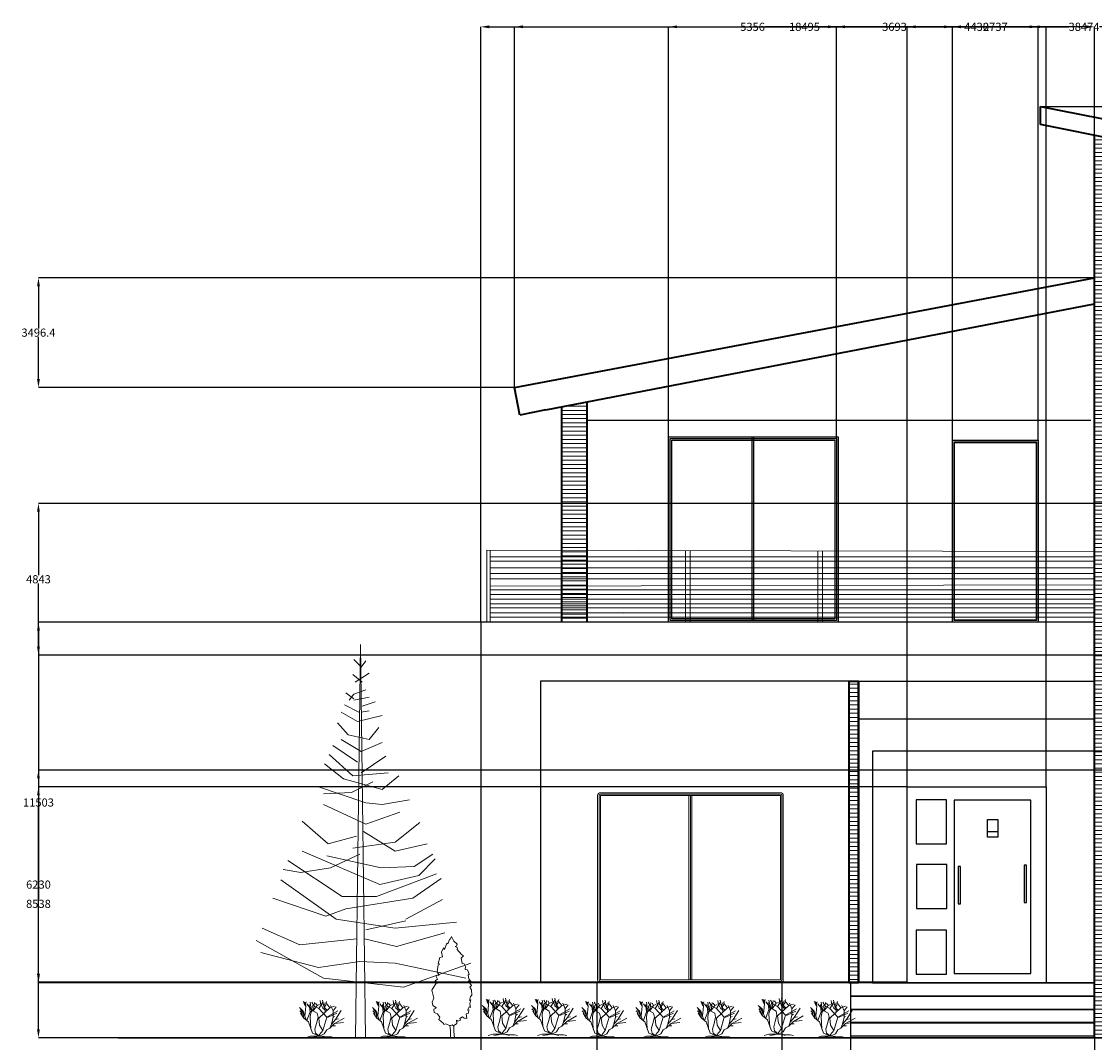
# Model space of a CAD drawing. Units: millimetres. Extents: x 23 to 3809233, y 4 to 290343.
# Tile 7 of 8: x 1887648 to 1921861, y 173128 to 205695. Entities that reach past the tile are written whole.
import ezdxf

# ---------------------------------------------------------------- set-up
doc = ezdxf.new("R2010")
doc.units = ezdxf.units.MM
doc.header["$MEASUREMENT"] = 0
for name, color, linetype, lineweight in [('A-ANNO-DIMS', 2, 'Continuous', 18), ('A-COLS', 7, 'Continuous', 35), ('A-DOOR', 3, 'Continuous', 25), ('A-ELEV', 7, 'Continuous', 25), ('A-ELEV-GRND', 7, 'Continuous', 30), ('A-FLOR-RAIL', 8, 'Continuous', 18), ('A-FLOR-STRS', 7, 'Continuous', 25), ('A-GLAZ', 4, 'Continuous', 18), ('A-ROOF', 7, 'Continuous', 35), ('A-WALL-PATT', 252, 'Continuous', 13), ('L-PLNT', 94, 'Continuous', 13)]:
    doc.layers.add(name, color=color, linetype=linetype, lineweight=lineweight)
doc.styles.get("Standard").update_dxf_attribs({"font": 'arial.ttf'})
doc.dimstyles.get("Standard").update_dxf_attribs({"dimtxt": 260.18, "dimasz": 270.18, "dimexe": 0.18, "dimexo": 0.0625, "dimgap": 0.09, "dimtad": 0, "dimtih": 1, "dimtoh": 1, "dimdec": 0, "dimzin": 0, "dimdsep": 46, "dimtxsty": 'Standard', "dimcen": 0.09, "dimadec": 0, "dimazin": 0, "dimtfac": 1, "dimtdec": 0, "dimtofl": 0, "dimtmove": 0, "dimatfit": 3, "dimfxl": 1, "dimtolj": 1, "dimtzin": 0, "dimarcsym": 0})

# ---------------------------------------------------------------- blocks, each defined once
blk = doc.blocks.new('*U6')
blk.add_lwpolyline([(-2.754, 191.699), (-6.78, 182.851), (-13.682, 176.953), (-11.956, 173.266), (-9.656, 172.529), (-14.257, 170.317), (-13.682, 167.368), (-21.733, 157.783), (-25.184, 154.834), (-21.158, 150.41), (-21.733, 147.461), (-22.884, 140.825), (-26.334, 140.087), (-29.21, 134.926), (-28.635, 129.028), (-32.661, 128.291), (-36.111, 120.18), (-34.386, 118.706), (-35.536, 111.333), (-38.987, 106.171), (-34.386, 107.646), (-40.712, 98.798), (-37.261, 95.849), (-40.712, 90.688), (-41.287, 80.366), (-38.412, 78.154), (-36.686, 70.781), (-39.562, 71.518), (-37.261, 64.145), (-38.412, 57.509), (-36.111, 58.247), (-33.236, 52.348), (-35.536, 53.086), (-34.961, 46.45), (-30.36, 44.975), (-31.51, 36.128), (-26.334, 36.865), (-23.459, 39.814), (-18.283, 36.128), (-20.008, 33.178), (-14.832, 31.704), (-11.956, 33.178), (-12.531, 27.28), (-6.205, 22.856), (-3.905, 24.331), (0.121, 22.856), (8.173, 26.543), (11.624, 25.068), (12.199, 27.28), (21.4, 34.653), (19.675, 39.077), (23.701, 44.975), (30.027, 47.924), (30.602, 53.823), (25.426, 56.772), (32.903, 61.196), (34.053, 67.094), (30.602, 75.205), (34.628, 89.951), (26.576, 103.222), (23.701, 103.222), (28.302, 107.646), (23.701, 110.595), (26.576, 115.756), (25.426, 117.968), (20.825, 118.706), (24.276, 124.604), (22.551, 137.876), (19.1, 139.35), (22.551, 140.825), (19.675, 151.884), (14.499, 153.359), (16.224, 162.207), (12.199, 170.317), (10.473, 167.368), (5.872, 179.165), (4.147, 177.69), (0.696, 187.275), (-0.454, 185.8)], close=True)
for points in [[(-6.813, 23.669), (-6.813, 11.669), (-8.627, 0)], [(0.387, 23.669), (-0.576, 13.271), (-0.576, 3.686), (0, 0)]]:
    blk.add_lwpolyline(points)
blk = doc.blocks.new('*U8')
for p, q in [((-2.401, 192), (-4.8, 0)), ((-2.401, 192), (0, 0)), ((-4.988, 183.92), (-2.688, 180.971)), ((-3.263, 186.869), (0.188, 186.869)), ((-2.113, 181.708), (0.763, 184.657)), ((-6.714, 178.022), (0.188, 173.598)), ((-3.263, 173.598), (1.338, 177.284)), ((-4.988, 169.911), (0.763, 167.699)), ((0.763, 165.487), (4.788, 168.437)), ((0.763, 167.699), (3.063, 164.75)), ((-3.263, 161.801), (-9.59, 164.013)), ((-6.714, 166.225), (0.763, 164.75)), ((-1.538, 158.852), (5.364, 162.538)), ((-0.963, 154.428), (-13.04, 157.377)), ((-6.714, 159.589), (-2.688, 158.852)), ((7.089, 158.852), (-0.963, 154.428)), ((-42.371, 67.426), (-24.542, 57.841)), ((-24.542, 57.104), (-4.988, 52.68)), ((27.218, 45.307), (45.622, 53.417)), ((-43.521, 51.205), (-19.942, 44.569)), ((-19.942, 44.569), (-4.413, 48.256)), ((-0.388, 48.256), (27.218, 45.307))]:
    blk.add_line(p, q)
for points in [[(8.814, 153.691), (3.638, 147.792), (-6.714, 145.58), (-11.315, 151.479)], [(-13.04, 144.106), (-2.688, 139.682), (7.089, 145.58)], [(-0.963, 134.521), (11.115, 142.631)], [(-15.916, 129.36), (1.338, 127.885), (12.84, 138.207)], [(-14.766, 137.47), (-2.688, 129.36)], [(-21.092, 127.885), (-13.04, 121.249), (5.939, 126.41), (15.141, 133.783)], [(-26.268, 116.088), (-13.04, 113.876), (-4.988, 114.613), (18.591, 122.724)], [(-8.439, 124.936), (1.913, 119.775), (15.716, 119.037)], [(-21.667, 110.19), (-4.988, 104.291), (15.716, 113.876)], [(-31.444, 105.028), (-19.366, 95.443), (1.338, 92.494)], [(-0.388, 98.393), (13.415, 94.706), (26.068, 105.766)], [(-34.895, 94.706), (-19.366, 91.02), (-3.838, 100.605)], [(-38.92, 87.333), (-30.869, 79.223), (-11.89, 74.799), (26.068, 91.02)], [(-37.77, 89.545), (-28.568, 83.647), (-12.465, 82.909), (13.99, 88.808)], [(-2.113, 89.545), (12.265, 82.909), (26.643, 80.697), (35.27, 82.172)], [(-39.496, 79.96), (-10.165, 68.901), (6.514, 68.901), (32.969, 86.596)], [(-49.272, 56.366), (-19.366, 53.417), (9.389, 57.841), (36.42, 77.011)], [(-41.796, 77.748), (-27.993, 68.163), (4.788, 63.002), (14.565, 59.316), (40.446, 68.163)], [(-56.174, 36.459), (-23.392, 24.662), (15.716, 29.086), (48.497, 47.519)], [(-53.873, 29.086), (-19.366, 36.459), (-2.113, 37.196), (18.016, 34.247), (46.197, 41.62)]]:
    blk.add_lwpolyline(points)
blk = doc.blocks.new('*U7')
for p, q in [((-16.8, 16.32), (-15.36, 19.68)), ((-14.88, 18.24), (-12.96, 20.64)), ((-12.471, 19.775), (-12.898, 22.044)), ((-11.677, 19.071), (-12.471, 19.775)), ((-11.28, 19.619), (-12.104, 21.184)), ((-11.921, 18.836), (-10.64, 20.401)), ((-11.433, 18.289), (-10.457, 22.749)), ((-10.579, 18.054), (-9.846, 19.697)), ((-8.16, 17.76), (-10.56, 21.6)), ((-9.48, 19.775), (-8.992, 22.592)), ((-7.2, 19.68), (-8.64, 20.16)), ((-7.2, 19.68), (-6.24, 21.12)), ((-4.8, 16.32), (-7.2, 19.68)), ((-5.086, 17.741), (-5.513, 21.34)), ((-5.28, 19.2), (-3.84, 21.6)), ((-2.88, 12.96), (-4.32, 19.68)), ((-3.84, 16.8), (-0.96, 20.64)), ((-3.377, 18.602), (-2.888, 21.575)), ((-2.88, 15.84), (-2.4, 20.16)), ((-0.508, 21.888), (-0.081, 20.558)), ((-0.203, 19.149), (0.102, 21.34)), ((-0.142, 19.384), (0.59, 20.401)), ((-0.02, 20.01), (0.896, 21.105)), ((0.041, 20.714), (1.384, 22.044)), ((0.102, 21.34), (0.835, 21.888)), ((-18.24, 11.04), (-21.755, 16.655)), ((-12.96, 12.48), (-19.68, 16.32)), ((-13.92, 12.48), (-19.2, 14.88)), ((-16.8, 16.32), (-18.72, 18.72)), ((-14.88, 18.24), (-17.76, 19.2)), ((-16.8, 12.48), (-16.8, 16.32)), ((-8.16, 12), (-14.88, 18.24)), ((-13.325, 16.724), (-11.433, 18.289)), ((-12.96, 12.48), (-8.16, 17.76)), ((-12.043, 15.628), (-11.921, 18.836)), ((-11.982, 16.802), (-10.579, 18.054)), ((-8.16, 17.76), (-5.28, 19.2)), ((-7.68, 12.48), (-7.2, 14.88)), ((-7.2, 14.88), (-3.84, 16.8)), ((-3.377, 15.315), (-5.086, 17.819)), ((-2.766, 16.802), (-3.377, 18.602)), ((-0.96, 10.56), (-2.88, 15.84)), ((-0.48, 10.8), (0.346, 13.203)), ((0.346, 13.203), (-0.203, 19.149)), ((0.346, 13.203), (1.323, 16.254)), ((0.96, 12), (1.44, 15.36)), ((0.96, 12), (2.88, 14.88)), ((1.323, 16.254), (3.642, 18.289)), ((1.44, 15.36), (2.88, 17.28)), ((1.92, 13.44), (2.4, 15.36)), ((2.4, 15.36), (3.36, 16.32)), ((-17.76, 8.64), (-23.663, 11.961)), ((-17.76, 8.64), (-23.128, 9.222)), ((-18.24, 11.04), (-20.16, 11.52)), ((-15.84, 8.16), (-18.24, 11.04)), ((-16.32, 7.2), (-18.24, 7.2)), ((-16.8, 12.48), (-17.76, 12.96)), ((-14.88, 5.76), (-17.76, 8.64)), ((-15.84, 8.16), (-16.8, 12.48)), ((-14.88, 5.76), (-15.84, 8.16)), ((-12.96, 12.48), (-13.92, 12.48)), ((-10.56, 4.32), (-12.96, 12.48)), ((-10.56, 4.32), (-8.64, 7.68)), ((-8.64, 7.68), (-8.16, 12)), ((-6.72, 8.64), (-7.68, 12.48)), ((-5.76, 5.28), (-6.72, 8.64)), ((-4.32, 2.88), (-1.92, 9.6)), ((-3.36, 5.28), (-2.88, 12.96)), ((-1.92, 9.6), (0.96, 12)), ((-15.84, 0.48), (-17.76, 0)), ((-13.44, 0.48), (-15.84, 0.48)), ((-12.96, 4.8), (-14.88, 5.76)), ((-9.6, 0.96), (-13.44, 0.48)), ((-11.52, 2.4), (-12.96, 4.8)), ((-9.6, 0.96), (-12.96, 0)), ((-8.64, 0.96), (-11.52, 2.4)), ((-8.64, 1.92), (-10.56, 4.32)), ((-9.6, 0.96), (-7.68, 0.96)), ((-8.64, 0.96), (-4.32, 2.88)), ((-8.64, 0.96), (-6.24, 2.88)), ((-8.64, 0.96), (-8.64, 1.92)), ((-8.64, 0.96), (-2.88, 0.96)), ((-7.68, 0.96), (-6.24, 0.48)), ((-6.24, 2.88), (-5.76, 5.28)), ((-6.24, 0.48), (-3.36, 0)), ((-2.88, 0.96), (0, 0))]:
    blk.add_line(p, q)
blk = doc.blocks.new('*D94')
at = {"layer": 'A-ANNO-DIMS', "color": 0, "lineweight": -2, "transparency": 16777216}
for p, q in [((1902289, 186535), (1902289, 205525)), ((1902560, 205524), (1921037, 205524)), ((1940493, 205524), (1922015, 205524)), ((1940763, 198959), (1940763, 205525))]:
    blk.add_line(p, q, dxfattribs=at)
at = {"layer": 'A-ANNO-DIMS', "color": 0, "transparency": 16777216}
for points in [[(1902560, 205569), (1902560, 205479), (1902289, 205524)], [(1940493, 205569), (1940493, 205479), (1940763, 205524)]]:
    blk.add_solid(points, dxfattribs=at)
at = {"layer": 'Defpoints', "color": 0, "transparency": 16777216}
for p in [(1940763, 205524), (1940763, 198959), (1902289, 186535)]:
    blk.add_point(p, dxfattribs=at)
at = {"layer": 'A-ANNO-DIMS', "color": 0, "transparency": 16777216, "insert": (1921526, 205524), "char_height": 260.2, "attachment_point": 5}
blk.add_mtext('\\A1;38474', dxfattribs=at)
blk = doc.blocks.new('*D95')
at = {"layer": 'A-ANNO-DIMS', "color": 0, "lineweight": -2, "transparency": 16777216}
for p, q in [((1920137, 202978), (1944019, 202978)), ((1944019, 202708), (1944019, 188263)), ((1944019, 173551), (1944019, 187997)), ((1939891, 173281), (1944019, 173281))]:
    blk.add_line(p, q, dxfattribs=at)
at = {"layer": 'A-ANNO-DIMS', "color": 0, "transparency": 16777216}
for points in [[(1943974, 202708), (1944064, 202708), (1944019, 202978)], [(1943974, 173551), (1944064, 173551), (1944019, 173281)]]:
    blk.add_solid(points, dxfattribs=at)
at = {"layer": 'Defpoints', "color": 0, "transparency": 16777216}
for p in [(1920137, 202978), (1944019, 202978), (1939891, 173281)]:
    blk.add_point(p, dxfattribs=at)
at = {"layer": 'A-ANNO-DIMS', "color": 0, "transparency": 16777216, "insert": (1944019, 188130), "char_height": 260.2, "attachment_point": 5}
blk.add_mtext('\\A1;29698', dxfattribs=at)
blk = doc.blocks.new('*D96')
at = {"layer": 'A-ANNO-DIMS', "color": 0, "lineweight": -2, "transparency": 16777216}
for p, q in [((1902289, 175032), (1902289, 166038)), ((1905995, 175031), (1905995, 166038)), ((1902560, 166038), (1903754, 166038)), ((1905725, 166038), (1904531, 166038))]:
    blk.add_line(p, q, dxfattribs=at)
at = {"layer": 'A-ANNO-DIMS', "color": 0, "transparency": 16777216}
for points in [[(1902560, 166083), (1902560, 165993), (1902289, 166038)], [(1905725, 166083), (1905725, 165993), (1905995, 166038)]]:
    blk.add_solid(points, dxfattribs=at)
at = {"layer": 'Defpoints', "color": 0, "transparency": 16777216}
for p in [(1902289, 175032), (1905995, 175031), (1905995, 166038)]:
    blk.add_point(p, dxfattribs=at)
at = {"layer": 'A-ANNO-DIMS', "color": 0, "transparency": 16777216, "insert": (1904142, 166038), "char_height": 260.2, "attachment_point": 5}
blk.add_mtext('\\A1;3706', dxfattribs=at)
blk = doc.blocks.new('*D97')
at = {"layer": 'A-ANNO-DIMS', "color": 0, "lineweight": -2, "transparency": 16777216}
for p, q in [((1905995, 175031), (1905995, 166038)), ((1911896, 175048), (1911896, 166038)), ((1906265, 166038), (1908582, 166038)), ((1911626, 166038), (1909309, 166038))]:
    blk.add_line(p, q, dxfattribs=at)
at = {"layer": 'A-ANNO-DIMS', "color": 0, "transparency": 16777216}
for points in [[(1906265, 166083), (1906265, 165993), (1905995, 166038)], [(1911626, 166083), (1911626, 165993), (1911896, 166038)]]:
    blk.add_solid(points, dxfattribs=at)
at = {"layer": 'Defpoints', "color": 0, "transparency": 16777216}
for p in [(1905995, 175031), (1911896, 175048), (1911896, 166038)]:
    blk.add_point(p, dxfattribs=at)
at = {"layer": 'A-ANNO-DIMS', "color": 0, "transparency": 16777216, "insert": (1908945, 166038), "char_height": 260.2, "attachment_point": 5}
blk.add_mtext('\\A1;5901', dxfattribs=at)
blk = doc.blocks.new('*D98')
at = {"layer": 'A-ANNO-DIMS', "color": 0, "lineweight": -2, "transparency": 16777216}
for p, q in [((1911896, 175048), (1911896, 166038)), ((1914080, 175026), (1914080, 166038)), ((1912166, 166038), (1912598, 166038)), ((1913810, 166038), (1913378, 166038))]:
    blk.add_line(p, q, dxfattribs=at)
at = {"layer": 'A-ANNO-DIMS', "color": 0, "transparency": 16777216}
for points in [[(1912166, 166083), (1912166, 165993), (1911896, 166038)], [(1913810, 166083), (1913810, 165993), (1914080, 166038)]]:
    blk.add_solid(points, dxfattribs=at)
at = {"layer": 'Defpoints', "color": 0, "transparency": 16777216}
for p in [(1911896, 175048), (1914080, 175026), (1914080, 166038)]:
    blk.add_point(p, dxfattribs=at)
at = {"layer": 'A-ANNO-DIMS', "color": 0, "transparency": 16777216, "insert": (1912988, 166038), "char_height": 260.2, "attachment_point": 5}
blk.add_mtext('\\A1;2184', dxfattribs=at)
blk = doc.blocks.new('*D102')
at = {"layer": 'A-ANNO-DIMS', "color": 0, "lineweight": -2, "transparency": 16777216}
for p, q in [((1914079.851314, 175025.824019), (1914079.851314, 166037.51032)), ((1921856.95103, 175025.824019), (1921856.95103, 166037.51032)), ((1914350.031314, 166037.69032), (1917580.88079, 166037.69032)), ((1921586.77103, 166037.69032), (1918355.921554, 166037.69032))]:
    blk.add_line(p, q, dxfattribs=at)
at = {"layer": 'A-ANNO-DIMS', "color": 0, "transparency": 16777216}
for points in [[(1914350.031314, 166082.72032), (1914350.031314, 165992.66032), (1914079.851314, 166037.69032)], [(1921586.77103, 166082.72032), (1921586.77103, 165992.66032), (1921856.95103, 166037.69032)]]:
    blk.add_solid(points, dxfattribs=at)
at = {"layer": 'Defpoints', "color": 0, "transparency": 16777216}
for p in [(1914079.851314, 175025.886519), (1921856.95103, 175025.886519), (1921856.95103, 166037.69032)]:
    blk.add_point(p, dxfattribs=at)
at = {"layer": 'A-ANNO-DIMS', "color": 0, "transparency": 16777216, "insert": (1917968.401172, 166037.69032), "char_height": 260.18, "attachment_point": 5}
blk.add_mtext('\\A1;7777', dxfattribs=at)
blk = doc.blocks.new('*D103')
at = {"layer": 'A-ANNO-DIMS', "color": 0, "lineweight": -2, "transparency": 16777216}
for p, q in [((1902289.331647, 186534.824099), (1888189.886131, 186534.824099)), ((1888190.066131, 186264.644099), (1888190.066131, 180916.359871)), ((1888190.066131, 175302.036407), (1888190.066131, 180650.320635)), ((1902289.331647, 175031.856407), (1888189.886131, 175031.856407))]:
    blk.add_line(p, q, dxfattribs=at)
at = {"layer": 'A-ANNO-DIMS', "color": 0, "transparency": 16777216}
for points in [[(1888145.036131, 186264.644099), (1888235.096131, 186264.644099), (1888190.066131, 186534.824099)], [(1888145.036131, 175302.036407), (1888235.096131, 175302.036407), (1888190.066131, 175031.856407)]]:
    blk.add_solid(points, dxfattribs=at)
at = {"layer": 'Defpoints', "color": 0, "transparency": 16777216}
for p in [(1888190.066131, 186534.824099), (1902289.394147, 186534.824099), (1902289.394147, 175031.856407)]:
    blk.add_point(p, dxfattribs=at)
at = {"layer": 'A-ANNO-DIMS', "color": 0, "transparency": 16777216, "insert": (1888190.066131, 180783.340253), "char_height": 260.18, "attachment_point": 5}
blk.add_mtext('\\A1;11503', dxfattribs=at)
blk = doc.blocks.new('*D104')
at = {"layer": 'A-ANNO-DIMS', "color": 0, "lineweight": -2, "transparency": 16777216}
for p, q in [((1924370.307623, 181820.425276), (1888189.886131, 181820.425276)), ((1888190.066131, 181550.245276), (1888190.066131, 177684.406757)), ((1888190.066131, 173552.529002), (1888190.066131, 177418.367521)), ((1924370.346212, 173282.349002), (1888189.886131, 173282.349002))]:
    blk.add_line(p, q, dxfattribs=at)
at = {"layer": 'A-ANNO-DIMS', "color": 0, "transparency": 16777216}
for points in [[(1888145.036131, 181550.245276), (1888235.096131, 181550.245276), (1888190.066131, 181820.425276)], [(1888145.036131, 173552.529002), (1888235.096131, 173552.529002), (1888190.066131, 173282.349002)]]:
    blk.add_solid(points, dxfattribs=at)
at = {"layer": 'Defpoints', "color": 0, "transparency": 16777216}
for p in [(1888190.066131, 181820.425276), (1924370.370123, 181820.425276), (1924370.408712, 173282.349002)]:
    blk.add_point(p, dxfattribs=at)
at = {"layer": 'A-ANNO-DIMS', "color": 0, "transparency": 16777216, "insert": (1888190.066131, 177551.387139), "char_height": 260.18, "attachment_point": 5}
blk.add_mtext('\\A1;8538', dxfattribs=at)
blk = doc.blocks.new('*D105')
at = {"layer": 'A-ANNO-DIMS', "color": 0, "lineweight": -2, "transparency": 16777216}
for p, q in [((1903366, 194022), (1903366, 205525)), ((1903636, 205524), (1912135, 205524)), ((1921591, 205524), (1913092, 205524)), ((1921861, 197518), (1921861, 205525))]:
    blk.add_line(p, q, dxfattribs=at)
at = {"layer": 'A-ANNO-DIMS', "color": 0, "transparency": 16777216}
for points in [[(1903636, 205569), (1903636, 205479), (1903366, 205524)], [(1921591, 205569), (1921591, 205479), (1921861, 205524)]]:
    blk.add_solid(points, dxfattribs=at)
at = {"layer": 'Defpoints', "color": 0, "transparency": 16777216}
for p in [(1921861, 205524), (1921861, 197518), (1903366, 194022)]:
    blk.add_point(p, dxfattribs=at)
at = {"layer": 'A-ANNO-DIMS', "color": 0, "transparency": 16777216, "insert": (1912613, 205524), "char_height": 260.2, "attachment_point": 5}
blk.add_mtext('\\A1;18495', dxfattribs=at)
blk = doc.blocks.new('*D107')
at = {"layer": 'A-ANNO-DIMS', "color": 0, "lineweight": -2, "transparency": 16777216}
for p, q in [((1921861, 197518), (1888190, 197518)), ((1888190, 197248), (1888190, 195903)), ((1888190, 194292), (1888190, 195637)), ((1903366, 194022), (1888190, 194022))]:
    blk.add_line(p, q, dxfattribs=at)
at = {"layer": 'A-ANNO-DIMS', "color": 0, "transparency": 16777216}
for points in [[(1888145, 197248), (1888235, 197248), (1888190, 197518)], [(1888145, 194292), (1888235, 194292), (1888190, 194022)]]:
    blk.add_solid(points, dxfattribs=at)
at = {"layer": 'Defpoints', "color": 0, "transparency": 16777216}
for p in [(1888190, 197518), (1921861, 197518), (1903366, 194022)]:
    blk.add_point(p, dxfattribs=at)
at = {"layer": 'A-ANNO-DIMS', "color": 0, "transparency": 16777216, "insert": (1888190, 195770), "char_height": 260.2, "attachment_point": 5}
blk.add_mtext('\\A1;3496.4', dxfattribs=at)
blk = doc.blocks.new('*D108')
at = {"layer": 'A-ANNO-DIMS', "color": 0, "lineweight": -2, "transparency": 16777216}
for p, q in [((1915886, 181281), (1915886, 205525)), ((1916157, 205524), (1917708, 205524)), ((1920046, 205524), (1918495, 205524)), ((1920317, 181281), (1920317, 205525))]:
    blk.add_line(p, q, dxfattribs=at)
at = {"layer": 'A-ANNO-DIMS', "color": 0, "transparency": 16777216}
for points in [[(1916157, 205569), (1916157, 205479), (1915886, 205524)], [(1920046, 205569), (1920046, 205479), (1920317, 205524)]]:
    blk.add_solid(points, dxfattribs=at)
at = {"layer": 'Defpoints', "color": 0, "transparency": 16777216}
for p in [(1920317, 205524), (1915886, 181281), (1920317, 181281)]:
    blk.add_point(p, dxfattribs=at)
at = {"layer": 'A-ANNO-DIMS', "color": 0, "transparency": 16777216, "insert": (1918101, 205524), "char_height": 260.2, "attachment_point": 5}
blk.add_mtext('\\A1;4430', dxfattribs=at)
blk = doc.blocks.new('*D109')
at = {"layer": 'A-ANNO-DIMS', "color": 0, "lineweight": -2, "transparency": 16777216}
for p, q in [((1915886, 181281), (1888190, 181281)), ((1888190, 181011), (1888190, 178299)), ((1888190, 175321), (1888190, 178033)), ((1915875, 175051), (1888190, 175051))]:
    blk.add_line(p, q, dxfattribs=at)
at = {"layer": 'A-ANNO-DIMS', "color": 0, "transparency": 16777216}
for points in [[(1888145, 181011), (1888235, 181011), (1888190, 181281)], [(1888145, 175321), (1888235, 175321), (1888190, 175051)]]:
    blk.add_solid(points, dxfattribs=at)
at = {"layer": 'Defpoints', "color": 0, "transparency": 16777216}
for p in [(1888190, 181281), (1915886, 181281), (1915875, 175051)]:
    blk.add_point(p, dxfattribs=at)
at = {"layer": 'A-ANNO-DIMS', "color": 0, "transparency": 16777216, "insert": (1888190, 178166), "char_height": 260.2, "attachment_point": 5}
blk.add_mtext('\\A1;6230', dxfattribs=at)
blk = doc.blocks.new('*D110')
at = {"layer": 'A-ANNO-DIMS', "color": 0, "lineweight": -2, "transparency": 16777216}
for p, q in [((1908280, 192442), (1908280, 205525)), ((1908550, 205524), (1910569, 205524)), ((1913366, 205524), (1911346, 205524)), ((1913636, 192391), (1913636, 205525))]:
    blk.add_line(p, q, dxfattribs=at)
at = {"layer": 'A-ANNO-DIMS', "color": 0, "transparency": 16777216}
for points in [[(1908550, 205569), (1908550, 205479), (1908280, 205524)], [(1913366, 205569), (1913366, 205479), (1913636, 205524)]]:
    blk.add_solid(points, dxfattribs=at)
at = {"layer": 'Defpoints', "color": 0, "transparency": 16777216}
for p in [(1913636, 205524), (1908280, 192442), (1913636, 192391)]:
    blk.add_point(p, dxfattribs=at)
at = {"layer": 'A-ANNO-DIMS', "color": 0, "transparency": 16777216, "insert": (1910958, 205524), "char_height": 260.2, "attachment_point": 5}
blk.add_mtext('\\A1;5356', dxfattribs=at)
blk = doc.blocks.new('*D111')
at = {"layer": 'A-ANNO-DIMS', "color": 0, "lineweight": -2, "transparency": 16777216}
for p, q in [((1913636, 192391), (1913636, 205525)), ((1913906, 205524), (1915094, 205524)), ((1917059, 205524), (1915871, 205524)), ((1917329, 192335), (1917329, 205525))]:
    blk.add_line(p, q, dxfattribs=at)
at = {"layer": 'A-ANNO-DIMS', "color": 0, "transparency": 16777216}
for points in [[(1913906, 205569), (1913906, 205479), (1913636, 205524)], [(1917059, 205569), (1917059, 205479), (1917329, 205524)]]:
    blk.add_solid(points, dxfattribs=at)
at = {"layer": 'Defpoints', "color": 0, "transparency": 16777216}
for p in [(1917329, 205524), (1913636, 192391), (1917329, 192335)]:
    blk.add_point(p, dxfattribs=at)
at = {"layer": 'A-ANNO-DIMS', "color": 0, "transparency": 16777216, "insert": (1915482, 205524), "char_height": 260.2, "attachment_point": 5}
blk.add_mtext('\\A1;3693', dxfattribs=at)
blk = doc.blocks.new('*D112')
at = {"layer": 'A-ANNO-DIMS', "color": 0, "lineweight": -2, "transparency": 16777216}
for p, q in [((1917329, 192335), (1917329, 205525)), ((1917599, 205524), (1918307, 205524)), ((1919796, 205524), (1919088, 205524)), ((1920066, 192336), (1920066, 205525))]:
    blk.add_line(p, q, dxfattribs=at)
at = {"layer": 'A-ANNO-DIMS', "color": 0, "transparency": 16777216}
for points in [[(1917599, 205569), (1917599, 205479), (1917329, 205524)], [(1919796, 205569), (1919796, 205479), (1920066, 205524)]]:
    blk.add_solid(points, dxfattribs=at)
at = {"layer": 'Defpoints', "color": 0, "transparency": 16777216}
for p in [(1920066, 205524), (1917329, 192335), (1920066, 192336)]:
    blk.add_point(p, dxfattribs=at)
at = {"layer": 'A-ANNO-DIMS', "color": 0, "transparency": 16777216, "insert": (1918698, 205524), "char_height": 260.2, "attachment_point": 5}
blk.add_mtext('\\A1;2737', dxfattribs=at)
blk = doc.blocks.new('*D115')
at = {"layer": 'A-ANNO-DIMS', "color": 0, "lineweight": -2, "transparency": 16777216}
for p, q in [((1929050.318541, 190325.231012), (1888189.886131, 190325.231012)), ((1888190.066131, 190055.051012), (1888190.066131, 188036.972999)), ((1888190.066131, 185752.85575), (1888190.066131, 187770.933763)), ((1929050.318541, 185482.67575), (1888189.886131, 185482.67575))]:
    blk.add_line(p, q, dxfattribs=at)
at = {"layer": 'A-ANNO-DIMS', "color": 0, "transparency": 16777216}
for points in [[(1888145.036131, 190055.051012), (1888235.096131, 190055.051012), (1888190.066131, 190325.231012)], [(1888145.036131, 185752.85575), (1888235.096131, 185752.85575), (1888190.066131, 185482.67575)]]:
    blk.add_solid(points, dxfattribs=at)
at = {"layer": 'Defpoints', "color": 0, "transparency": 16777216}
for p in [(1888190.066131, 190325.231012), (1929050.381041, 190325.231012), (1929050.381041, 185482.67575)]:
    blk.add_point(p, dxfattribs=at)
at = {"layer": 'A-ANNO-DIMS', "color": 0, "transparency": 16777216, "insert": (1888190.066131, 187903.953381), "char_height": 260.18, "attachment_point": 5}
blk.add_mtext('\\A1;4843', dxfattribs=at)

msp = doc.modelspace()

# ---------------------------------------------------------------- hatches: boundary and pattern name
at = {"layer": 'A-WALL-PATT'}
h = msp.add_hatch(dxfattribs=at)
h.set_pattern_fill('ANSI31', color=256, scale=1061.3134, angle=-45, style=0)
h.paths.add_polyline_path([(1921860.931, 182422.235), (1925481.709, 182422.235), (1925481.709, 201356.818), (1921860.931, 202063.759)])
h.paths.add_polyline_path([(1922672.309, 192384.187), (1924806.696, 192384.187), (1924806.696, 186534.824), (1922672.309, 186534.824)], flags=0)
h = msp.add_hatch(dxfattribs=at)
h.set_pattern_fill('ANSI31', color=256, scale=1061.3134, angle=-45, style=0)
h.paths.add_polyline_path([(1904871.979, 186534.824), (1905677.267, 186534.824), (1905677.267, 193557.268), (1904871.979, 193401.456)])
h = msp.add_hatch(dxfattribs=at)
h.set_pattern_fill('ANSI31', color=256, scale=1061.3134, angle=-45, style=0)
h.paths.add_polyline_path([(1921860.931, 173280.749), (1923056.615, 173280.749), (1923056.615, 182422.235), (1921860.931, 182422.235)])

# ---------------------------------------------------------------- linework, layer by layer
at = {"layer": 'A-COLS'}
for p, q in [((1921860.931, 197729.802), (1921860.931, 202063.759)), ((1921860.931, 193396.712), (1921860.931, 197729.802)), ((1904871.979, 186534.824), (1904871.979, 193401.456)), ((1905677.267, 193557.268), (1905677.267, 186534.824)), ((1921860.931, 173280.749), (1921860.931, 193396.712)), ((1921860.931, 182422.235), (1925481.709, 182422.235))]:
    msp.add_line(p, q, dxfattribs=at)
msp.add_lwpolyline([(1914330.122, 175031.856, -0.414213562), (1914328.132, 175029.866), (1914038.151, 175029.866, -0.414213562), (1914036.161, 175031.856), (1914036.161, 184646.818, -0.414213562), (1914038.151, 184648.808), (1914328.132, 184648.808, -0.414213562), (1914330.122, 184646.818)], format="xyb", close=True, dxfattribs=at)
at = {"layer": 'A-DOOR'}
for p, q in [((1910930.32, 192444.023), (1910930.32, 186587.89)), ((1910983.385, 192444.023), (1910983.385, 186587.89)), ((1918449.576, 179860.536), (1918782.108, 179860.536))]:
    msp.add_line(p, q, dxfattribs=at)
for points in [[(1913688.902, 186536.814, -0.414213562), (1913686.912, 186534.824), (1908279.859, 186534.824, -0.414213562), (1908277.869, 186536.814), (1908277.869, 192442.033, -0.414213562), (1908279.859, 192444.023), (1913686.912, 192444.023, -0.414213562), (1913688.902, 192442.033)], [(1920068.178, 186536.814, -0.414213562), (1920066.188, 186534.824), (1917330.981, 186534.824, -0.414213562), (1917328.991, 186536.814), (1917328.991, 192334.119, -0.414213562), (1917330.981, 192336.109), (1920066.188, 192336.109, -0.414213562), (1920068.178, 192334.119)], [(1915886.417, 181281.405, -0.414213562), (1915888.407, 181283.395), (1920316.559, 181283.395, -0.414213562), (1920318.549, 181281.405), (1920318.549, 175029.866, -0.414213562), (1920316.559, 175027.876), (1915888.407, 175027.876, -0.414213562), (1915886.417, 175029.866)], [(1917140.668, 180868.352, 0.414213562), (1917138.679, 180870.342), (1916175.947, 180870.342, 0.414213562), (1916173.957, 180868.352), (1916173.957, 179470.983, 0.414213562), (1916175.947, 179468.993), (1917138.679, 179468.993, 0.414213562), (1917140.668, 179470.983)], [(1919834.377, 180856.261, 0.414213562), (1919832.387, 180858.251), (1917382.944, 180858.251, 0.414213562), (1917380.954, 180856.261), (1917380.954, 175334.38, 0.414213562), (1917382.944, 175332.39), (1919832.387, 175332.39, 0.414213562), (1919834.377, 175334.38)], [(1918449.576, 180239.005, -0.414213562), (1918451.566, 180240.995), (1918780.118, 180240.995, -0.414213562), (1918782.108, 180239.005), (1918782.108, 179675.165, -0.414213562), (1918780.118, 179673.175), (1918451.566, 179673.175, -0.414213562), (1918449.576, 179675.165)], [(1917151.659, 178800.765, 0.414213562), (1917149.669, 178802.755), (1916186.938, 178802.755, 0.414213562), (1916184.948, 178800.765), (1916184.948, 177403.396, 0.414213562), (1916186.938, 177401.406), (1917149.669, 177401.406, 0.414213562), (1917151.659, 177403.396)], [(1917587.674, 178739.103, 0.414213562), (1917585.684, 178741.093), (1917514.577, 178741.093, 0.414213562), (1917512.587, 178739.103), (1917512.587, 177553.876, 0.414213562), (1917514.577, 177551.886), (1917585.684, 177551.886, 0.414213562), (1917587.674, 177553.876)], [(1919693.052, 178781.957, 0.414213562), (1919691.062, 178783.947), (1919619.954, 178783.947, 0.414213562), (1919617.964, 178781.957), (1919617.964, 177596.73, 0.414213562), (1919619.954, 177594.74), (1919691.062, 177594.74, 0.414213562), (1919693.052, 177596.73)], [(1917140.668, 176711.934, 0.414213562), (1917138.679, 176713.924), (1916175.947, 176713.924, 0.414213562), (1916173.957, 176711.934), (1916173.957, 175314.565, 0.414213562), (1916175.947, 175312.575), (1917138.679, 175312.575, 0.414213562), (1917140.668, 175314.565)]]:
    msp.add_lwpolyline(points, format="xyb", close=True, dxfattribs=at)
for points in [[(1913635.836, 186587.89), (1908330.934, 186587.89), (1908330.934, 192390.957), (1913635.836, 192390.957)], [(1913582.771, 186640.955), (1908384, 186640.955), (1908384, 192337.892), (1913582.771, 192337.892)], [(1920015.112, 186587.89), (1917382.057, 186587.89), (1917382.057, 192283.044), (1920015.112, 192283.044)], [(1920001.845, 186601.156), (1917395.323, 186601.156), (1917395.323, 192269.777), (1920001.845, 192269.777)]]:
    msp.add_lwpolyline(points, close=True, dxfattribs=at)
at = {"layer": 'A-ELEV'}
for p, q in [((1921746.04, 192969.037), (1905677.267, 192969.037)), ((1921860.931, 186534.824), (1902289.394, 186534.824)), ((1902289.394, 186534.824), (1902289.394, 175031.856)), ((1914038.151, 184648.808), (1904201.652, 184648.808)), ((1904201.652, 184648.808), (1904201.652, 175031.856)), ((1914328.132, 183451.741), (1921860.931, 183451.741)), ((1914036.161, 175031.856), (1901938.029, 175031.856))]:
    msp.add_line(p, q, dxfattribs=at)
for points in [[(1921860.931, 175029.866, -0.414213562), (1921858.941, 175027.876), (1914330.122, 175027.876, -0.414213562), (1914328.132, 175029.866), (1914328.132, 184649.141, -0.414213562), (1914330.122, 184651.131), (1921858.941, 184651.131, -0.414213562), (1921860.931, 184649.141)], [(1921860.931, 182420.245, 0.414213562), (1921858.941, 182422.235), (1914788.488, 182422.235, 0.414213562), (1914786.498, 182420.245), (1914786.498, 175029.866, 0.414213562), (1914788.488, 175027.876), (1921858.941, 175027.876, 0.414213562), (1921860.931, 175029.866)]]:
    msp.add_lwpolyline(points, format="xyb", close=True, dxfattribs=at)
at = {"layer": 'A-ELEV-GRND'}
for p, q in [((1897673.161, 173280.749), (1890736.066, 173280.749)), ((1914495.5, 173280.749), (1897673.161, 173280.749)), ((1914495.5, 173280.749), (1941473.027, 173280.749))]:
    msp.add_line(p, q, dxfattribs=at)
at = {"layer": 'A-FLOR-RAIL'}
for p, q in [((1902481.163, 186534.824), (1902481.163, 188828.726)), ((1902481.163, 188828.726), (1921860.931, 188790.115)), ((1902593.408, 188828.502), (1902593.408, 186534.824)), ((1902593.408, 188622.773), (1921860.931, 188622.773)), ((1908824.05, 188816.089), (1908824.05, 186534.824)), ((1908973.44, 188815.791), (1908973.44, 186534.824)), ((1913039.967, 188816.089), (1913039.967, 186534.824)), ((1913189.356, 188815.791), (1913189.356, 186534.824)), ((1902593.408, 188478.136), (1921860.931, 188478.136)), ((1902593.408, 188263.358), (1921860.931, 188263.358)), ((1902593.408, 188084.974), (1921860.931, 188084.974)), ((1902593.408, 187918.43), (1921860.931, 187918.43)), ((1902593.408, 187681.663), (1921860.931, 187728.802)), ((1902593.408, 187569.564), (1921860.931, 187569.564)), ((1902593.408, 187422.12), (1921860.931, 187422.12)), ((1902593.408, 187269.466), (1921860.931, 187269.466)), ((1902593.408, 187122.888), (1921860.931, 187122.888)), ((1902593.408, 186991.511), (1921860.931, 186991.511)), ((1902593.408, 186835.926), (1921860.931, 186835.926)), ((1902593.408, 186693.495), (1921860.931, 186693.495))]:
    msp.add_line(p, q, dxfattribs=at)
at = {"layer": 'A-FLOR-STRS'}
for points in [[(1921858.941, 175025.887, 0.414213562), (1921856.951, 175027.876), (1914079.851, 175027.876, 0.414213562), (1914077.861, 175025.887), (1914077.861, 174605.46, 0.414213562), (1914079.851, 174603.47), (1921856.951, 174603.47, 0.414213562), (1921858.941, 174605.46)], [(1921858.941, 174603.47, 0.414213562), (1921856.951, 174605.46), (1914079.851, 174605.46, 0.414213562), (1914077.861, 174603.47), (1914077.861, 174183.043, 0.414213562), (1914079.851, 174181.053), (1921856.951, 174181.053, 0.414213562), (1921858.941, 174183.043)], [(1921856.951, 174183.043, 0.414213562), (1921854.961, 174185.033), (1914077.861, 174185.033, 0.414213562), (1914075.871, 174183.043), (1914075.871, 173762.616, 0.414213562), (1914077.861, 173760.626), (1921854.961, 173760.626, 0.414213562), (1921856.951, 173762.616)], [(1921856.948, 173760.626, 0.414213562), (1921854.958, 173762.616), (1914077.858, 173762.616, 0.414213562), (1914075.868, 173760.626), (1914075.868, 173340.199, 0.414213562), (1914077.858, 173338.209), (1921854.958, 173338.209, 0.414213562), (1921856.948, 173340.199)]]:
    msp.add_lwpolyline(points, format="xyb", close=True, dxfattribs=at)
at = {"layer": 'A-GLAZ'}
for p, q in [((1908930.816, 181004.392), (1908930.816, 175124.721)), ((1908977.249, 181004.392), (1908977.249, 175124.721)), ((1909023.681, 181004.392), (1909023.681, 175124.721))]:
    msp.add_line(p, q, dxfattribs=at)
for points in [[(1906016.874, 175126.711, 0.414213562), (1906111.729, 175031.856), (1911842.769, 175031.856, 0.414213562), (1911937.624, 175126.711), (1911937.624, 181002.402, 0.414213562), (1911842.769, 181097.257), (1906111.729, 181097.257, 0.414213562), (1906016.874, 181002.402)], [(1906063.306, 175126.711, 0.414213562), (1906111.729, 175078.289), (1911842.769, 175078.289, 0.414213562), (1911891.191, 175126.711), (1911891.191, 181002.402, 0.414213562), (1911842.769, 181050.824), (1906111.729, 181050.824, 0.414213562), (1906063.306, 181002.402)], [(1906109.739, 175126.711, 0.414213562), (1906111.729, 175124.721), (1911842.769, 175124.721, 0.414213562), (1911844.759, 175126.711), (1911844.759, 181002.402, 0.414213562), (1911842.769, 181004.392), (1906111.729, 181004.392, 0.414213562), (1906109.739, 181002.402)]]:
    msp.add_lwpolyline(points, format="xyb", close=True, dxfattribs=at)
at = {"layer": 'A-ROOF'}
for p, q in [((1920136.86, 202413.849), (1920136.86, 202978.465)), ((1920136.86, 202978.465), (1940762.989, 198959.058)), ((1940749.627, 198207.142), (1920136.86, 202413.849)), ((1903365.563, 194021.715), (1921860.931, 197518.123)), ((1904365.122, 193303.386), (1921860.931, 196688.585)), ((1903535.604, 193142.885), (1903365.563, 194021.715)), ((1904365.122, 193303.386), (1903535.604, 193142.885))]:
    msp.add_line(p, q, dxfattribs=at)
at = {"layer": 'A-WALL-PATT'}
msp.add_line((1906845.408, 186802.841), (1906845.408, 186802.841), dxfattribs=at)
for points in [[(1914036.161, 184559.299), (1914328.132, 184559.299)], [(1914036.161, 184426.635), (1914328.132, 184426.635)], [(1914036.161, 184293.971), (1914328.132, 184293.971)], [(1914036.161, 184161.307), (1914328.132, 184161.307)], [(1914036.161, 184028.643), (1914328.132, 184028.643)], [(1914036.161, 183895.978), (1914328.132, 183895.978)], [(1914036.161, 183763.314), (1914328.132, 183763.314)], [(1914036.161, 183630.65), (1914328.132, 183630.65)], [(1914036.161, 183497.986), (1914328.132, 183497.986)], [(1914036.161, 183365.322), (1914328.132, 183365.322)], [(1914036.161, 183232.657), (1914328.132, 183232.657)], [(1914036.161, 183099.993), (1914328.132, 183099.993)], [(1914036.161, 182967.329), (1914328.132, 182967.329)], [(1914036.161, 182834.665), (1914328.132, 182834.665)], [(1914036.161, 182702.001), (1914328.132, 182702.001)], [(1914036.161, 182569.337), (1914328.132, 182569.337)], [(1914036.161, 182436.672), (1914328.132, 182436.672)], [(1914036.161, 182304.008), (1914328.132, 182304.008)], [(1914036.161, 182171.344), (1914328.132, 182171.344)], [(1914036.161, 182038.68), (1914328.132, 182038.68)], [(1914036.161, 181906.016), (1914328.132, 181906.016)], [(1914036.161, 181773.352), (1914328.132, 181773.352)], [(1914036.161, 181640.687), (1914328.132, 181640.687)], [(1914036.161, 181508.023), (1914328.132, 181508.023)], [(1914036.161, 181375.359), (1914328.132, 181375.359)], [(1914036.161, 181242.695), (1914328.132, 181242.695)], [(1914036.161, 181110.031), (1914328.132, 181110.031)], [(1914036.161, 180977.367), (1914328.132, 180977.367)], [(1914036.161, 180844.702), (1914328.132, 180844.702)], [(1914036.161, 180712.038), (1914328.132, 180712.038)], [(1914036.161, 180579.374), (1914328.132, 180579.374)], [(1914036.161, 180446.71), (1914328.132, 180446.71)], [(1914036.161, 180314.046), (1914328.132, 180314.046)], [(1914036.161, 180181.382), (1914328.132, 180181.382)], [(1914036.161, 180048.717), (1914328.132, 180048.717)], [(1914036.161, 179916.053), (1914328.132, 179916.053)], [(1914036.161, 179783.389), (1914328.132, 179783.389)], [(1914036.161, 179650.725), (1914328.132, 179650.725)], [(1914036.161, 179518.061), (1914328.132, 179518.061)], [(1914036.161, 179385.396), (1914328.132, 179385.396)], [(1914036.161, 179252.732), (1914328.132, 179252.732)], [(1914036.161, 179120.068), (1914328.132, 179120.068)], [(1914036.161, 178987.404), (1914328.132, 178987.404)], [(1914036.161, 178854.74), (1914328.132, 178854.74)], [(1914036.161, 178722.076), (1914328.132, 178722.076)], [(1914036.161, 178589.411), (1914328.132, 178589.411)], [(1914036.161, 178456.747), (1914328.132, 178456.747)], [(1914036.161, 178324.083), (1914328.132, 178324.083)], [(1914036.161, 178191.419), (1914328.132, 178191.419)], [(1914036.161, 178058.755), (1914328.132, 178058.755)], [(1914036.161, 177926.091), (1914328.132, 177926.091)], [(1914036.161, 177793.426), (1914328.132, 177793.426)], [(1914036.161, 177660.762), (1914328.132, 177660.762)], [(1914036.161, 177528.098), (1914328.132, 177528.098)], [(1914036.161, 177395.434), (1914328.132, 177395.434)], [(1914036.161, 177262.77), (1914328.132, 177262.77)], [(1914036.161, 177130.106), (1914328.132, 177130.106)], [(1914036.161, 176997.441), (1914328.132, 176997.441)], [(1914036.161, 176864.777), (1914328.132, 176864.777)], [(1914036.161, 176732.113), (1914328.132, 176732.113)], [(1914036.161, 176599.449), (1914328.132, 176599.449)], [(1914036.161, 176466.785), (1914328.132, 176466.785)], [(1914036.161, 176334.12), (1914328.132, 176334.12)], [(1914036.161, 176201.456), (1914328.132, 176201.456)], [(1914036.161, 176068.792), (1914328.132, 176068.792)], [(1914036.161, 175936.128), (1914328.132, 175936.128)], [(1914036.161, 175803.464), (1914328.132, 175803.464)], [(1914036.161, 175670.8), (1914328.132, 175670.8)], [(1914036.161, 175538.135), (1914328.132, 175538.135)], [(1914036.161, 175405.471), (1914328.132, 175405.471)], [(1914036.161, 175272.807), (1914328.132, 175272.807)], [(1914036.161, 175140.143), (1914328.132, 175140.143)]]:
    msp.add_lwpolyline(points, dxfattribs=at)

# ---------------------------------------------------------------- block references
at = {"layer": 'L-PLNT'}
for name, p, xscale, yscale, zscale in [('*U8', (1898300.213, 173280.749), -65.33947381132158, 65.33947381132158, 65.33947381132158), ('*U6', (1901313.96, 173280.749), -16.84835000712546, 16.84835000712546, 16.84835000712546), ('*U7', (1902532.364, 173348.158), -52.46997559542009, 52.46997559542009, 52.46997559542009), ('*U7', (1904099.866, 173348.158), -52.46997559542009, 52.46997559542009, 52.46997559542009), ('*U7', (1911329.807, 173348.158), -52.46997559542009, 52.46997559542009, 52.46997559542009), ('*U7', (1896699.838, 173280.749), -52.46997559542009, 52.46997559542009, 52.46997559542009), ('*U7', (1899028.267, 173280.749), -52.46997559542009, 52.46997559542009, 52.46997559542009), ('*U7', (1905704.752, 173280.749), -52.46997559542009, 52.46997559542009, 52.46997559542009), ('*U7', (1907425.527, 173280.749), -52.46997559542009, 52.46997559542009, 52.46997559542009), ('*U7', (1909377.667, 173280.749), -52.46997559542009, 52.46997559542009, 52.46997559542009), ('*U7', (1912992.74, 173280.749), -52.46997559542009, 52.46997559542009, 52.46997559542009)]:
    msp.add_blockref(name, p, dxfattribs=dict(at, xscale=xscale, yscale=yscale, zscale=zscale))

# ---------------------------------------------------------------- dimensions: what is measured, and where the dimension line sits
at = {"layer": 'A-ANNO-DIMS'}
for base, p1, p2, picture, middle in [((1940762.989, 205524.465), (1902289.394, 186534.824), (1940762.989, 198959.058), '*D94', (1921526.192, 205524.465)), ((1921860.931, 205524.465), (1903365.563, 194021.715), (1921860.931, 197518.123), '*D105', (1912613.247, 205524.465)), ((1913635.836, 205524.465), (1908279.859, 192442.033), (1913635.836, 192390.957), '*D110', (1910957.847, 205524.465)), ((1917329.147, 205524.465), (1913635.836, 192390.957), (1917329.147, 192334.894), '*D111', (1915482.492, 205524.465)), ((1920316.559, 205524.465), (1915886.417, 181281.405), (1920316.559, 181281.405), '*D108', (1918101.488, 205524.465)), ((1920066.188, 205524.465), (1917329.147, 192334.894), (1920066.188, 192336.109), '*D112', (1918697.667, 205524.465)), ((1905995.105, 166037.69), (1902289.394, 175031.856), (1905995.105, 175031.011), '*D96', (1904142.249, 166037.69)), ((1911895.803, 166037.69), (1905995.105, 175031.011), (1911895.803, 175048.056), '*D97', (1908945.454, 166037.69)), ((1914079.851, 166037.69), (1911895.803, 175048.056), (1914079.851, 175025.887), '*D98', (1912987.827, 166037.69)), ((1921856.951, 166037.69), (1914079.851, 175025.887), (1921856.951, 175025.887), '*D102', (1917968.401, 166037.69))]:
    dim = msp.add_linear_dim(base=base, p1=p1, p2=p2, dimstyle='Standard', override={"dimdec": 0, "dimlfac": 1, "dimrnd": 0, "dimzin": 0, "dimdsep": 46, "dimlunit": 2}, dxfattribs=at)
    dim.commit()
    dim.dimension.update_dxf_attribs({"geometry": picture, "text_midpoint": middle})
for base, p1, p2, override, picture, middle in [((1944019.027, 202978.465), (1939891.392, 173280.749), (1920136.86, 202978.465), {"dimdec": 0, "dimlfac": 1, "dimrnd": 0, "dimzin": 0, "dimdsep": 46, "dimlunit": 2}, '*D95', (1944019.027, 188129.607)), ((1888190.066, 197518.123), (1903365.563, 194021.715), (1921860.931, 197518.123), {"dimdec": 1, "dimlfac": 1, "dimrnd": 0, "dimzin": 0, "dimdsep": 46, "dimlunit": 2}, '*D107', (1888190.066, 195769.919)), ((1888190.066, 190325.231), (1929050.381, 185482.676), (1929050.381, 190325.231), {"dimdec": 0, "dimlfac": 1, "dimrnd": 0, "dimzin": 0, "dimdsep": 46, "dimlunit": 2}, '*D115', (1888190.066, 187903.953)), ((1888190.066, 186534.824), (1902289.394, 175031.856), (1902289.394, 186534.824), {"dimdec": 0, "dimlfac": 1, "dimrnd": 0, "dimzin": 0, "dimdsep": 46, "dimlunit": 2}, '*D103', (1888190.066, 180783.34)), ((1888190.066, 181820.425), (1924370.409, 173282.349), (1924370.37, 181820.425), {"dimdec": 0, "dimlfac": 1, "dimrnd": 0, "dimzin": 0, "dimdsep": 46, "dimlunit": 2}, '*D104', (1888190.066, 177551.387)), ((1888190.066, 181281.405), (1915874.863, 175051.243), (1915886.417, 181281.405), {"dimdec": 0, "dimlfac": 1, "dimrnd": 0, "dimzin": 0, "dimdsep": 46, "dimlunit": 2}, '*D109', (1888190.066, 178166.324))]:
    dim = msp.add_linear_dim(base=base, p1=p1, p2=p2, angle=90, dimstyle='Standard', override=override, dxfattribs=at)
    dim.commit()
    dim.dimension.update_dxf_attribs({"geometry": picture, "text_midpoint": middle})

doc.saveas('drawing.dxf')
